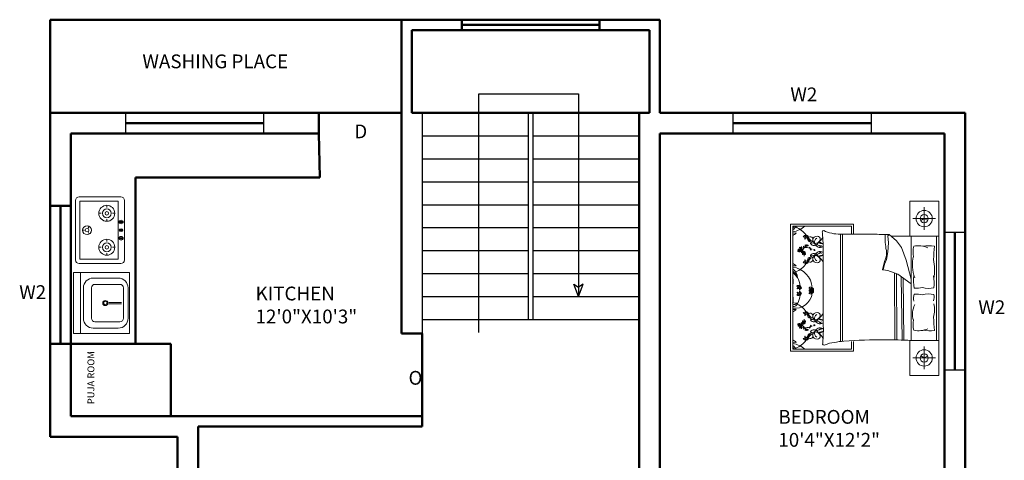
# Model space of a CAD drawing. Units: inches. Extents: x 18 to 447, y -515 to 49.
# Tile 2 of 2: x 18 to 447, y -143 to 49. Entities that reach past the tile are written whole.
import ezdxf

# ---------------------------------------------------------------- set-up
doc = ezdxf.new("R2010")
doc.units = ezdxf.units.IN
doc.header["$MEASUREMENT"] = 0
for name, color, linetype, lineweight in [('A-ANNO-TEXT', 7, 'Continuous', 25), ('A-AREA-IDEN', 3, 'Continuous', 25), ('A-FLOR-FIXT', 9, 'Continuous', 18), ('A-FLOR-STRS', 3, 'Continuous', 25), ('A-FURN', 8, 'Continuous', 18), ('A-GLAZ', 4, 'Continuous', 25), ('A-WALL', 7, 'Continuous', 50)]:
    doc.layers.add(name, color=color, linetype=linetype, lineweight=lineweight)
doc.styles.get("Standard").update_dxf_attribs({"font": 'arial.ttf'})

# ---------------------------------------------------------------- blocks, each defined once
blk = doc.blocks.new('М14 600х655')
for p, q in [((-655, 600), (-655, 0)), ((-655, 600), (-655, 0)), ((-655, 0), (-655, 600)), ((0, 600), (-655, 600)), ((0, 0), (0, 600)), ((0, 525), (-655, 525)), ((-165, 494), (-490, 494)), ((-596, 388), (-596, 121)), ((-528, 370), (-528, 103)), ((-165, 408), (-490, 408)), ((-127, 103), (-127, 370)), ((-59, 121), (-59, 388)), ((-334, 87), (-334, 220)), ((-321, 87), (-321, 220)), ((-655, 0), (-655, 0)), ((-655, 0), (-655, 0)), ((-655, 0), (0, 0)), ((-655, 0), (0, 0)), ((-490, 65), (-165, 65)), ((-490, 15), (-165, 15))]:
    blk.add_line(p, q)
for radius in [27.6, 19.3]:
    blk.add_circle((-327, 259), radius)
for centre, radius, start, end in [((-490, 388), 106, 90, 180), ((-165, 388), 106, 0, 90), ((-490, 370), 38.2, 90, 180), ((-165, 370), 38.2, 0, 90), ((-490, 121), 106, 180, 270), ((-165, 121), 106, 270, 0), ((-490, 103), 38.2, 180, 270), ((-165, 103), 38.2, 270, 0)]:
    blk.add_arc(centre, radius, start, end)
blk = doc.blocks.new('BED-DOUBLE')
for p, q in [((412.28, -42.96), (412.28, -33.06)), ((418.6, -30.43), (418.6, -106.23)), ((407.33, -38.01), (417.24, -38.01)), ((354.14, -40.44), (381.44, -40.44)), ((354.14, -95.69), (354.14, -40.44)), ((355.02, -41.31), (355.02, -94.82)), ((380.57, -41.31), (355.02, -41.31)), ((380.57, -44.72), (380.57, -41.31)), ((381.44, -40.44), (381.44, -44.72)), ((375.77, -91.48), (375.77, -44.72)), ((376.72, -91.41), (376.72, -44.72)), ((396.39, -45.53), (397.01, -44.91)), ((396.7, -48.6), (396.39, -45.53)), ((397.01, -44.91), (400.23, -47.67)), ((418.6, -45.59), (397.8, -45.59)), ((406.62, -45.59), (406.62, -91.07)), ((417.63, -91.07), (417.63, -45.59)), ((362.7, -48.78), (363.56, -48.62)), ((396.39, -52.43), (396.7, -48.6)), ((400.23, -47.67), (402.37, -50.59)), ((402.37, -50.59), (404.37, -56.12)), ((362.7, -54.08), (363.56, -54.25)), ((368.33, -83.72), (368.33, -52.94)), ((395.93, -55.81), (396.39, -52.43)), ((394.4, -60.26), (395.01, -57.81)), ((395.01, -57.81), (395.93, -55.81)), ((404.37, -56.12), (406.62, -64.38)), ((396.39, -60.57), (394.4, -60.26)), ((400.84, -62.26), (396.39, -60.57)), ((399.53, -90.8), (399.41, -61.72)), ((400.31, -90.8), (400.19, -62.01)), ((406.62, -66.41), (400.84, -62.26)), ((402.7, -90.83), (402.31, -63.31)), ((403.47, -90.86), (403.1, -63.88)), ((362.7, -82.05), (363.56, -81.88)), ((362.7, -87.35), (363.56, -87.51)), ((380.57, -94.82), (380.57, -91.47)), ((381.44, -91.49), (381.44, -95.69)), ((412.28, -93.7), (412.28, -103.6)), ((381.44, -95.69), (354.14, -95.69)), ((355.02, -94.82), (380.57, -94.82)), ((407.33, -98.65), (417.24, -98.65))]:
    blk.add_line(p, q)
for points in [[(405.97, -45.59), (405.97, -30.43), (418.6, -30.43)], [(412.28, -38.01), (410.75, -38.89)], [(412.28, -38.01), (413.82, -38.89)], [(418.6, -91.07), (405.97, -91.07), (405.97, -106.23), (418.6, -106.23)], [(412.28, -98.65), (410.75, -97.76)], [(412.28, -98.65), (413.82, -97.76)]]:
    blk.add_lwpolyline(points)
for points in [[(390.06, -44.75, 0.001242), (375.68, -44.72, -0.127202), (368.52, -43.2)], [(416.71, -49.94, 0.074897), (411.76, -50.04, -0.472817)], [(411.48, -67.97, 0.14099), (416.53, -68.13, 0.235245)], [(411.48, -71.21, -0.14099), (416.53, -71.06, -0.235245)], [(416.71, -86.71, -0.074897), (411.76, -86.62, 0.472817)], [(377.31, -91.39, 0.056112), (373.14, -91.94, 0.095341), (369.13, -93.01)]]:
    blk.add_lwpolyline(points, format="xyb")
for centre, radius in [((412.28, -38.01), 3.54), ((412.28, -38.01), 1.77), ((357.92, -51.9), 0.193), ((359.96, -53.16), 0.193), ((357.92, -84.23), 0.193), ((359.96, -82.97), 0.193), ((412.28, -98.65), 3.54), ((412.28, -98.65), 1.77)]:
    blk.add_circle(centre, radius)
for centre, radius, start, end in [((351.46, -37.17), 6.01, 306.3036, 316.4814), ((352.36, -38.91), 4.82, 303.4617, 330.1116), ((353.69, -33.94), 9.9, 277.745, 311.8856), ((352.71, -50.88), 9.9, 34.3865, 68.5908), ((353.48, -41.61), 4.02, 292.5547, 318.9546), ((355.64, -30.59), 13.69, 267.4081, 273.6519), ((360.64, -46.36), 1.1, 77.7115, 159.0387), ((360.05, -45.26), 0.827, 238.4633, 358.2869), ((362.76, -46.94), 2.5, 138.8402, 177.9352), ((360.38, -46.85), 0.123, 177.9352, 11.4834), ((360.44, -46.84), 0.0597, 11.4834, 127.9409), ((361.25, -46.01), 0.81, 117.6827, 223.7762), ((360.74, -46.49), 0.107, 223.7762, 159.7183), ((361.07, -46.09), 0.821, 2.9516, 103.728), ((367.63, -43.79), 6.92, 192.5173, 207.1824), ((359.96, -46.56), 1.56, 345.4653, 54.2343), ((362.32, -44.41), 1.69, 211.3827, 255.2969), ((362.98, -46.78), 1.42, 175.969, 254.3045), ((362.64, -47.05), 1.14, 350.264, 160.8688), ((361.41, -46.82), 0.697, 333.9755, 53.2681), ((361.1, -48.31), 1.51, 6.1662, 51.5825), ((365.15, -44.79), 3.58, 211.2614, 251.7045), ((365.56, -47.47), 1.81, 84.9449, 172.8857), ((366.25, -48.18), 1.76, 111.5819, 201.4221), ((364.8, -46.55), 2.28, 265.2933, 346.921), ((365.74, -46.94), 1.28, 354.4856, 91.0538), ((362.99, -43.6), 5.74, 303.6671, 333.2997), ((368.56, -43.89), 0.699, 93.98, 207.3412), ((289.43, -52.04), 78.9, 359.3433, 5.6887), ((395.12, 24.59), 69.52, 265.8294, 271.553), ((423.85, -46.21), 28.61, 177.4519, 191.3392), ((357.77, -51.51), 0.381, 157.4086, 261.4386), ((357.56, -51.49), 0.191, 58.0499, 135.6268), ((357.34, -51.85), 0.609, 14.7558, 58.0499), ((358.19, -51.69), 0.263, 36.1046, 181.4281), ((358.2, -50.65), 0.216, 124.3538, 214.3923), ((358.52, -50.69), 0.503, 190.3057, 287.1958), ((358.66, -50.51), 0.583, 176.9701, 248.2913), ((362.83, -47.43), 5.64, 212.6784, 216.3746), ((358.47, -50.64), 0.223, 216.3746, 291.7548), ((360.44, -53.78), 3.15, 124.0033, 132.4917), ((357.21, -54.17), 3.36, 63.7819, 68.2913), ((359, -51.59), 0.535, 128.3208, 208.8162), ((359, -50.8), 0.503, 122.8155, 187.3992), ((358.61, -51.01), 0.168, 289.3605, 111.7548), ((358.74, -51.01), 0.168, 221.8703, 44.2646), ((359.5, -51.5), 0.88, 157.2305, 229.0635), ((359.22, -50.86), 0.583, 109.4799, 177.6828), ((359.21, -51.21), 0.518, 174.4544, 220.6188), ((356.26, -54.1), 3.78, 30.544, 49.818), ((358.91, -50.49), 0.216, 56.8636, 146.9021), ((359.02, -50.73), 0.223, 148.8844, 224.2646), ((363.66, -53.53), 5.64, 145.1882, 148.8844), ((360.44, -53.78), 3.15, 94.756, 119.2041), ((367.14, -58.31), 10.36, 132.2412, 142.1744), ((361.92, -50.06), 2.14, 178.3264, 187.1302), ((359.61, -50.36), 0.398, 11.3256, 64.4621), ((360.96, -49.79), 1.2, 190.2588, 210.656), ((360.15, -50.28), 0.364, 188.3432, 274.2869), ((360.47, -50.07), 0.635, 210.656, 242.6341), ((360.95, -49.53), 1.22, 218.2101, 226.3071), ((360.05, -50.55), 0.154, 325.7657, 67.4417), ((355.26, -45.39), 7.2, 313.1541, 322.0459), ((360.6, -56.9), 6.28, 73.5842, 93.8277), ((360.55, -49.71), 0.148, 142.4737, 265.053), ((360.75, -49.68), 0.319, 127.7621, 169.0403), ((360.58, -49.41), 0.449, 265.053, 338.3618), ((361.17, -50.03), 0.586, 113.4276, 137.6104), ((361.1, -49.42), 0.193, 183.2768, 356.7232), ((361.25, -49.77), 0.316, 139.7889, 227.6792), ((361.15, -49.88), 0.166, 227.6792, 350.3487), ((360.5, -49.76), 0.632, 353.0852, 15.7171), ((360.92, -49.84), 0.399, 350.3487, 43.6538), ((361.66, -49.43), 0.464, 198.7263, 262.5032), ((361.29, -49.64), 0.184, 1.1081, 91.8675), ((361.63, -49.74), 0.149, 255.2356, 54.9248), ((361.4, -49.69), 0.322, 11.5637, 52.6358), ((364.47, -50.52), 2.14, 178.3264, 187.1302), ((362.16, -50.81), 0.398, 11.3256, 64.4621), ((363.51, -50.24), 1.2, 190.2588, 210.656), ((362.7, -50.73), 0.364, 188.3432, 274.2869), ((363.02, -50.53), 0.635, 210.656, 242.6341), ((363.5, -49.98), 1.22, 218.2101, 226.3071), ((364.86, -44.76), 4.07, 236.2883, 266.5076), ((362.6, -51), 0.154, 325.7657, 67.4417), ((363.04, -51.29), 0.364, 147.5332, 233.4768), ((364.34, -47.84), 1.88, 209.9085, 343.1337), ((363.37, -51.1), 0.635, 179.1859, 211.164), ((362.75, -51.24), 0.154, 354.3784, 96.0543), ((360.6, -56.9), 6.28, 63.0032, 69.8941), ((363.85, -50.81), 1.2, 211.164, 231.5612), ((364.07, -50.93), 1.22, 195.5129, 203.6099), ((362.71, -51.73), 0.398, 357.3579, 50.4944), ((365.96, -47.15), 2.2, 182.3591, 234.0401), ((365.13, -49.04), 0.47, 167.3041, 285.1471), ((366.4, -51.29), 2.92, 122.7011, 126.3445), ((366.95, -48.14), 2.42, 199.2822, 299.1751), ((365.66, -50.99), 1.55, 41.5653, 105.1471), ((367.77, -45.7), 3.14, 238.8218, 279.1554), ((366.4, -51.29), 2.92, 55.785, 94.7304), ((366.51, -47.77), 2.18, 277.436, 299.9149), ((367.67, -49.21), 1.13, 221.5653, 293.8354), ((367.49, -49.59), 0.913, 30.0293, 52.325), ((367.49, -49.59), 0.913, 314.4517, 333.558), ((417.6, -52.65), 10.16, 165.1039, 191.0369), ((409.77, -59.6), 9.77, 65.1316, 101.7583), ((1138.04, -91.72), 722.54, 176.68521, 177.14978), ((357.37, -52.19), 0.148, 142.4737, 265.053), ((357.56, -52.16), 0.319, 61.2196, 169.0403), ((357.4, -51.89), 0.449, 265.053, 338.3618), ((357.99, -52.51), 0.586, 113.4276, 137.6104), ((357.76, -51.61), 0.128, 172.906, 277.132), ((358.06, -52.25), 0.316, 139.7889, 227.6792), ((357.96, -52.36), 0.166, 227.6792, 350.3487), ((357.32, -52.24), 0.632, 353.0852, 15.7171), ((357.73, -52.32), 0.399, 350.3487, 43.6538), ((358.47, -51.91), 0.464, 198.7263, 262.5032), ((358.04, -51.48), 0.266, 270.0645, 331.1507), ((358.26, -51.54), 0.304, 221.8413, 265.7877), ((358.1, -52.12), 0.184, 1.1081, 91.8675), ((358.26, -51.66), 0.189, 263.7526, 41.7054), ((358.22, -52.17), 0.322, 11.5637, 86.365), ((358.45, -52.22), 0.149, 255.2356, 54.9248), ((359.1, -51.55), 0.639, 207.7043, 254.3516), ((358.68, -51.91), 0.88, 270.278, 342.111), ((359.27, -53.01), 0.622, 98.7227, 159.3375), ((358.96, -52.21), 0.639, 244.9899, 291.6373), ((358.34, -51.95), 0.622, 340.0041, 40.6188), ((359.1, -51.89), 0.518, 278.7227, 324.8872), ((359, -52.31), 0.535, 290.5253, 358.5375), ((359.4, -53.45), 0.148, 142.4737, 265.053), ((359.6, -53.42), 0.319, 61.2196, 169.0403), ((359.43, -53.16), 0.449, 265.053, 338.3618), ((359.81, -52.77), 0.381, 157.4086, 261.4386), ((359.59, -52.76), 0.191, 58.0499, 135.6268), ((360.05, -52.15), 0.535, 182.8499, 266.1226), ((359.84, -51.78), 0.518, 231.7607, 277.9252), ((360.24, -51.68), 0.88, 214.5369, 286.3699), ((360.02, -53.77), 0.586, 113.4276, 137.6104), ((359.79, -52.88), 0.128, 172.906, 277.132), ((359.37, -53.11), 0.609, 14.7558, 58.0499), ((356.26, -54.1), 3.78, 23.0501, 23.8477), ((360.1, -53.51), 0.316, 139.7889, 227.6792), ((360, -53.62), 0.166, 227.6792, 350.3487), ((360, -52.91), 0.622, 37.3105, 97.9252), ((360.23, -52.95), 0.263, 36.1046, 181.4281), ((359.35, -53.51), 0.632, 353.0852, 15.7171), ((360.07, -52.05), 0.639, 265.0106, 311.658), ((356.26, -54.1), 3.78, 357.1071, 4.7585), ((359.77, -53.58), 0.399, 350.3487, 43.6538), ((360.07, -52.74), 0.266, 270.0645, 331.1507), ((360.3, -52.8), 0.304, 221.8413, 265.7877), ((360.51, -53.17), 0.464, 198.7263, 262.5032), ((360.14, -53.39), 0.184, 1.1081, 91.8675), ((360.3, -52.92), 0.189, 263.7526, 41.7054), ((360.26, -53.43), 0.322, 11.5637, 86.365), ((360.49, -53.49), 0.149, 255.2356, 54.9248), ((362.98, -56.09), 1.42, 105.6955, 184.031), ((362.64, -55.81), 1.14, 199.1312, 9.736), ((361.1, -54.56), 1.51, 308.4175, 353.8338), ((365.15, -58.07), 3.58, 108.2955, 148.7386), ((364.86, -58.1), 4.07, 93.4924, 123.7117), ((364.34, -55.02), 1.88, 16.8663, 150.0915), ((364.06, -49.83), 2.14, 234.6898, 243.4936), ((365.96, -55.71), 2.2, 125.9599, 177.6409), ((365.56, -55.4), 1.81, 187.1143, 275.0551), ((364.42, -51.65), 0.146, 12.7051, 190.4384), ((364.51, -51.63), 0.238, 190.4384, 10.4136), ((366.25, -54.69), 1.76, 158.5779, 248.4181), ((364.8, -56.31), 2.28, 13.079, 94.7067), ((365.13, -53.83), 0.47, 74.8529, 192.6959), ((366.95, -54.73), 2.42, 60.8249, 160.7178), ((366.4, -51.58), 2.92, 233.6555, 237.2989), ((365.66, -51.87), 1.55, 254.8529, 318.4347), ((367.77, -57.16), 3.14, 79.7133, 121.1782), ((366.4, -51.58), 2.92, 265.2696, 304.215), ((362.99, -59.26), 5.74, 21.4941, 56.3329), ((366.51, -55.09), 2.18, 60.0851, 82.564), ((367.67, -53.66), 1.13, 66.1646, 138.4347), ((367.49, -53.27), 0.913, 307.675, 336.7144), ((367.49, -53.27), 0.913, 23.229, 45.5483), ((423.04, -65.53), 29.39, 160.1194, 169.3383), ((389.75, -53.05), 6.17, 336.2616, 11.3392), ((424.82, -57.99), 17.62, 168.0397, 199.2615), ((353.48, -61.25), 4.02, 41.0454, 67.4453), ((355.64, -72.28), 13.69, 86.3481, 92.5919), ((353.69, -68.92), 9.9, 4.4623, 82.255), ((352.36, -63.95), 4.82, 1.272, 56.5383), ((352.71, -51.98), 9.9, 291.4092, 325.6135), ((360.05, -57.6), 0.827, 1.7131, 121.5367), ((360.64, -56.5), 1.1, 200.9613, 282.2885), ((360.38, -56.01), 0.123, 348.5166, 182.0648), ((362.76, -55.93), 2.5, 182.0648, 221.1598), ((360.44, -56.03), 0.0597, 232.0591, 348.5166), ((361.25, -56.86), 0.81, 136.2238, 242.3173), ((360.78, -56.38), 0.0645, 200.2667, 136.2271), ((359.96, -56.3), 1.56, 305.7657, 14.5347), ((367.63, -59.08), 6.92, 152.8176, 167.4827), ((361.07, -56.78), 0.821, 256.272, 357.0484), ((362.32, -58.45), 1.69, 104.7031, 148.6173), ((361.41, -56.05), 0.697, 306.7319, 26.0245), ((365.74, -55.92), 1.28, 268.9462, 5.5144), ((389.28, -60.33), 27.49, 352.2196, 9.497), ((351.46, -65.69), 6.01, 17.8504, 53.6964), ((349.77, -68.85), 8.94, 34.0123, 54.053), ((349.81, -65.39), 5.44, 343.5431, 17.0202), ((348.38, -68.16), 9.9, 4.4623, 27.4146), ((394.34, -60.09), 0.183, 178.8623, 289.7536), ((420.97, -65.13), 13.37, 169.8617, 193.6238), ((403.18, -66.14), 13.51, 351.5249, 13.96), ((347.01, -67.55), 8.05, 4.3787, 5.6357), ((341.5, -71.79), 14.38, 19.7217, 19.9028), ((357.51, -68.2), 1.1, 47.7873, 129.1145), ((357.55, -66.96), 0.827, 208.5391, 328.3627), ((357.04, -68.5), 0.123, 148.011, 341.5592), ((359.06, -69.76), 2.5, 108.9159, 148.011), ((357.1, -68.52), 0.0597, 341.5592, 98.0167), ((358.22, -68.2), 0.81, 87.7585, 193.852), ((357.54, -68.37), 0.107, 193.852, 129.9245), ((364.86, -69.46), 6.92, 162.593, 177.2582), ((356.83, -68.03), 1.56, 315.5411, 24.3101), ((359.94, -67.35), 1.69, 181.4585, 225.3727), ((358.02, -68.18), 0.821, 333.0274, 73.8037), ((362.82, -68.96), 1.1, 47.7873, 129.1145), ((362.85, -67.71), 0.827, 208.5391, 328.3627), ((364.36, -70.52), 2.5, 108.9159, 148.011), ((363.52, -68.96), 0.81, 87.7585, 193.852), ((362.13, -68.79), 1.56, 315.5411, 24.3101), ((370.16, -70.22), 6.92, 162.593, 177.2582), ((363.32, -68.94), 0.821, 333.0274, 73.8037), ((365.24, -68.11), 1.69, 181.4585, 225.3727), ((408.95, -59.04), 9.29, 264.0129, 285.8293), ((355.97, -69.42), 7.66, 262.8636, 351.8197), ((349.81, -73.26), 5.44, 342.9798, 16.4569), ((347.01, -71.11), 8.05, 354.3643, 355.6213), ((341.5, -66.87), 14.38, 340.0972, 340.2783), ((357.55, -71.7), 0.827, 31.6373, 151.4609), ((357.51, -70.45), 1.1, 230.8855, 312.2127), ((357.04, -70.16), 0.123, 18.4408, 211.989), ((359.06, -68.9), 2.5, 211.989, 251.0841), ((357.1, -70.14), 0.0597, 261.9833, 18.4408), ((348.38, -70.5), 9.9, 332.5854, 355.5377), ((358.22, -70.46), 0.81, 166.148, 272.2415), ((357.58, -70.28), 0.0645, 230.1909, 166.0209), ((364.86, -69.19), 6.92, 182.7418, 197.407), ((356.83, -70.62), 1.56, 335.6899, 44.4589), ((359.94, -71.31), 1.69, 134.6273, 178.5415), ((358.02, -70.48), 0.821, 286.1963, 26.9726), ((362.85, -70.94), 0.827, 31.6373, 151.4609), ((362.82, -69.69), 1.1, 230.8855, 312.2127), ((362.35, -69.26), 0.123, 148.011, 341.5592), ((362.35, -69.4), 0.123, 18.4408, 211.989), ((364.36, -68.14), 2.5, 211.989, 251.0841), ((362.41, -69.28), 0.0597, 341.5592, 98.0167), ((362.41, -69.38), 0.0597, 261.9833, 18.4408), ((363.52, -69.7), 0.81, 166.148, 272.2415), ((362.84, -69.13), 0.107, 193.852, 129.9245), ((362.88, -69.52), 0.0645, 230.1909, 166.0209), ((362.13, -69.86), 1.56, 335.6899, 44.4589), ((370.16, -68.44), 6.92, 182.7418, 197.407), ((363.32, -69.72), 0.821, 286.1963, 26.9726), ((365.24, -70.55), 1.69, 134.6273, 178.5415), ((411.62, -72.61), 4.02, 155.0183, 198.5407), ((408.95, -80.15), 9.29, 74.1707, 95.9871), ((412.93, -72.1), 3.75, 333.3437, 16.1026), ((356.67, -70.41), 4.43, 248.117, 276.6195), ((355.44, -74.47), 1.78, 256.3898, 349.0739), ((355.68, -73.14), 2.25, 252.8609, 311.9049), ((352.71, -84.14), 9.9, 34.3865, 68.5908), ((416.85, -79.63), 9.65, 153.8761, 196.1746), ((403.45, -77.72), 13.32, 346.3427, 11.1841), ((355.64, -63.85), 13.69, 267.4081, 273.6519), ((353.48, -74.88), 4.02, 292.5547, 318.9546), ((360.64, -79.63), 1.1, 77.7115, 159.0387), ((360.05, -78.53), 0.827, 238.4633, 358.2869), ((362.76, -80.2), 2.5, 138.8402, 177.9352), ((360.38, -80.12), 0.123, 177.9352, 11.4834), ((360.44, -80.1), 0.0597, 11.4834, 127.9409), ((361.25, -79.27), 0.81, 117.6827, 223.7762), ((360.74, -79.76), 0.107, 223.7762, 159.7183), ((361.07, -79.35), 0.821, 2.9516, 103.728), ((362.32, -77.67), 1.69, 211.3827, 255.2969), ((359.96, -79.82), 1.56, 345.4653, 54.2343), ((367.63, -77.05), 6.92, 192.5173, 207.1824), ((362.98, -80.04), 1.42, 175.969, 254.3045), ((362.64, -80.32), 1.14, 350.264, 160.8688), ((361.41, -80.08), 0.697, 333.9755, 53.2681), ((361.1, -81.57), 1.51, 6.1662, 51.5825), ((365.15, -78.06), 3.58, 211.2614, 251.7045), ((364.86, -78.03), 4.07, 236.2883, 266.5076), ((365.56, -80.73), 1.81, 84.9449, 172.8857), ((365.96, -80.42), 2.2, 182.3591, 234.0401), ((366.25, -81.44), 1.76, 111.5819, 201.4221), ((364.8, -79.81), 2.28, 265.2933, 346.921), ((365.74, -80.21), 1.28, 354.4856, 91.0538), ((362.99, -76.87), 5.74, 303.6671, 338.5059), ((1138.04, -44.94), 722.54, 182.85022, 183.31479), ((357.37, -83.94), 0.148, 94.947, 217.5263), ((357.56, -83.97), 0.319, 190.9597, 298.7804), ((357.4, -84.24), 0.449, 21.6382, 94.947), ((357.77, -84.62), 0.381, 98.5614, 202.5914), ((357.56, -84.64), 0.191, 224.3732, 301.9501), ((357.99, -83.62), 0.586, 222.3896, 246.5724), ((357.76, -84.52), 0.128, 82.868, 187.094), ((357.34, -84.28), 0.609, 301.9501, 345.2442), ((358.06, -83.88), 0.316, 132.3208, 220.2111), ((357.96, -83.77), 0.166, 9.6513, 132.3208), ((357.32, -83.88), 0.632, 344.2829, 6.9148), ((358.19, -84.44), 0.263, 178.5719, 323.8954), ((358.2, -85.47), 0.216, 145.6077, 235.6462), ((357.73, -83.81), 0.399, 316.3462, 9.6513), ((358.47, -84.22), 0.464, 97.4968, 161.2737), ((358.52, -85.44), 0.503, 72.8042, 169.6943), ((358.26, -84.59), 0.304, 94.2123, 138.1587), ((358.04, -84.65), 0.266, 28.8493, 89.9355), ((358.66, -85.62), 0.583, 111.7087, 183.0299), ((362.83, -88.7), 5.64, 143.6254, 147.3216), ((358.1, -84), 0.184, 268.1325, 358.8919), ((358.22, -83.96), 0.322, 273.635, 348.4363), ((358.26, -84.47), 0.189, 318.2946, 96.2474), ((358.47, -85.49), 0.223, 68.2452, 143.6254), ((360.44, -82.35), 3.15, 227.5083, 235.9967), ((358.45, -83.91), 0.149, 305.0752, 104.7644), ((357.21, -81.96), 3.36, 291.7087, 296.2181), ((359, -84.54), 0.535, 151.1838, 231.6792), ((359, -85.33), 0.503, 172.6008, 237.1845), ((359.1, -84.58), 0.639, 105.6484, 152.2957), ((358.61, -85.12), 0.168, 248.2452, 70.6395), ((358.74, -85.12), 0.168, 315.7354, 138.1297), ((359.5, -84.63), 0.88, 130.9365, 202.7695), ((359.22, -85.26), 0.583, 182.3172, 250.5201), ((358.96, -83.92), 0.639, 68.3627, 115.0101), ((358.68, -84.22), 0.88, 17.889, 89.722), ((359.27, -83.12), 0.622, 200.6625, 261.2773), ((359.21, -84.92), 0.518, 139.3812, 185.5456), ((356.26, -82.03), 3.78, 310.182, 329.456), ((359.02, -85.39), 0.223, 135.7354, 211.1156), ((358.34, -84.18), 0.622, 319.3812, 19.9959), ((363.66, -82.6), 5.64, 211.1156, 214.8118), ((360.44, -82.35), 3.15, 240.7959, 265.244), ((367.14, -77.82), 10.36, 217.8256, 227.7588), ((359.1, -84.24), 0.518, 35.1128, 81.2773), ((359, -83.82), 0.535, 1.4625, 69.4747), ((359.4, -82.67), 0.148, 94.947, 217.5263), ((359.6, -82.7), 0.319, 190.9597, 298.7804), ((359.43, -82.97), 0.449, 21.6382, 94.947), ((359.81, -83.36), 0.381, 98.5614, 202.5914), ((359.59, -83.37), 0.191, 224.3732, 301.9501), ((360.05, -83.98), 0.535, 93.8774, 177.1501), ((360.24, -84.44), 0.88, 73.6301, 145.4631), ((359.84, -84.35), 0.518, 82.0748, 128.2393), ((360.02, -82.36), 0.586, 222.3896, 246.5724), ((359.79, -83.25), 0.128, 82.868, 187.094), ((359.37, -83.02), 0.609, 301.9501, 345.2442), ((356.26, -82.03), 3.78, 336.1523, 336.9499), ((360.1, -82.62), 0.316, 132.3208, 220.2111), ((360.96, -86.34), 1.2, 149.344, 169.7412), ((360.15, -85.85), 0.364, 85.7131, 171.6568), ((360, -82.51), 0.166, 9.6513, 132.3208), ((360, -83.22), 0.622, 262.0748, 322.6895), ((360.47, -86.05), 0.635, 117.3659, 149.344), ((359.35, -82.62), 0.632, 344.2829, 6.9148), ((360.23, -83.18), 0.263, 178.5719, 323.8954), ((360.95, -86.6), 1.22, 133.6929, 141.7899), ((360.07, -84.08), 0.639, 48.342, 94.9894), ((356.26, -82.03), 3.78, 355.2415, 2.8929), ((359.77, -82.55), 0.399, 316.3462, 9.6513), ((360.51, -82.96), 0.464, 97.4968, 161.2737), ((360.3, -83.32), 0.304, 94.2123, 138.1587), ((360.07, -83.39), 0.266, 28.8493, 89.9355), ((360.05, -85.58), 0.154, 292.5583, 34.2343), ((360.14, -82.74), 0.184, 268.1325, 358.8919), ((360.6, -79.23), 6.28, 266.1723, 286.4158), ((355.26, -90.74), 7.2, 37.9541, 46.8459), ((360.26, -82.7), 0.322, 273.635, 348.4363), ((360.3, -83.21), 0.189, 318.2946, 96.2474), ((360.49, -82.64), 0.149, 305.0752, 104.7644), ((363.51, -85.89), 1.2, 149.344, 169.7412), ((364.47, -85.61), 2.14, 172.8698, 181.6736), ((362.16, -85.32), 0.398, 295.5379, 348.6744), ((362.7, -85.4), 0.364, 85.7131, 171.6568), ((363.02, -85.6), 0.635, 117.3659, 149.344), ((363.5, -86.15), 1.22, 133.6929, 141.7899), ((362.6, -85.13), 0.154, 292.5583, 34.2343), ((363.04, -84.84), 0.364, 126.5232, 212.4668), ((364.34, -81.11), 1.88, 209.9085, 343.1337), ((363.37, -85.03), 0.635, 148.836, 180.8141), ((362.75, -84.88), 0.154, 263.9457, 5.6216), ((360.6, -79.23), 6.28, 290.1059, 296.9968), ((363.85, -85.32), 1.2, 128.4388, 148.836), ((364.06, -86.3), 2.14, 116.5064, 125.3102), ((364.07, -85.2), 1.22, 156.3901, 164.4871), ((362.71, -84.4), 0.398, 309.5056, 2.6421), ((364.51, -84.5), 0.238, 349.5864, 169.5616), ((364.42, -84.48), 0.146, 169.5616, 347.2949), ((365.13, -82.3), 0.47, 167.3041, 285.1471), ((366.4, -84.55), 2.92, 122.7011, 126.3445), ((366.95, -81.4), 2.42, 199.2822, 299.1751), ((366.95, -87.99), 2.42, 60.8249, 160.7178), ((365.66, -84.26), 1.55, 41.5653, 105.1471), ((367.77, -78.97), 3.14, 238.8218, 280.2867), ((366.4, -84.55), 2.92, 55.785, 94.7304), ((366.51, -81.04), 2.18, 277.436, 299.9149), ((367.67, -82.47), 1.13, 221.5653, 293.8354), ((367.49, -82.86), 0.913, 23.2856, 52.325), ((294.61, -86.04), 73.76, 355.2402, 1.8035), ((367.49, -82.86), 0.913, 314.4517, 336.7144), ((417.6, -84.01), 10.16, 168.9631, 194.8961), ((358.91, -85.63), 0.216, 213.0979, 303.1364), ((361.92, -86.07), 2.14, 172.8698, 181.6736), ((359.61, -85.77), 0.398, 295.5379, 348.6744), ((360.38, -89.28), 0.123, 348.5166, 182.0648), ((362.76, -89.19), 2.5, 182.0648, 221.1598), ((360.55, -86.42), 0.148, 94.947, 217.5263), ((360.44, -89.29), 0.0597, 232.0591, 348.5166), ((360.75, -86.45), 0.319, 190.9597, 232.2379), ((361.25, -90.12), 0.81, 136.2238, 242.3173), ((360.58, -86.72), 0.449, 21.6382, 94.947), ((360.78, -89.65), 0.0645, 200.2667, 136.2271), ((361.17, -86.1), 0.586, 222.3896, 246.5724), ((367.63, -92.34), 6.92, 152.8176, 167.4827), ((359.96, -89.57), 1.56, 305.7657, 14.5347), ((361.1, -86.71), 0.193, 3.2768, 176.7232), ((361.25, -86.36), 0.316, 132.3208, 220.2111), ((361.15, -86.25), 0.166, 9.6513, 132.3208), ((360.5, -86.36), 0.632, 344.2829, 6.9148), ((360.92, -86.29), 0.399, 316.3462, 9.6513), ((361.66, -86.7), 0.464, 97.4968, 161.2737), ((361.29, -86.48), 0.184, 268.1325, 358.8919), ((362.98, -89.35), 1.42, 105.6955, 184.031), ((362.64, -89.08), 1.14, 199.1312, 9.736), ((361.63, -86.38), 0.149, 305.0752, 104.7644), ((361.4, -86.44), 0.322, 307.3642, 348.4363), ((361.41, -89.31), 0.697, 306.7319, 26.0245), ((361.1, -87.82), 1.51, 308.4175, 353.8338), ((365.15, -91.34), 3.58, 108.2955, 148.7386), ((364.86, -91.37), 4.07, 93.4924, 123.7117), ((364.34, -88.29), 1.88, 16.8663, 150.0915), ((365.96, -88.98), 2.2, 125.9599, 177.6409), ((365.56, -88.66), 1.81, 187.1143, 275.0551), ((366.25, -87.95), 1.76, 158.5779, 248.4181), ((364.8, -89.58), 2.28, 13.079, 94.7067), ((365.13, -87.09), 0.47, 74.8529, 192.6959), ((366.4, -84.84), 2.92, 233.6555, 237.2989), ((365.66, -85.14), 1.55, 254.8529, 318.4347), ((365.74, -89.19), 1.28, 268.9462, 5.5144), ((367.77, -90.43), 3.14, 79.249, 121.1782), ((366.4, -84.84), 2.92, 265.2696, 304.215), ((362.99, -92.53), 5.74, 23.6453, 56.3329), ((366.51, -88.36), 2.18, 60.0851, 82.564), ((367.67, -86.92), 1.13, 66.1646, 138.4347), ((367.49, -86.54), 0.913, 307.675, 342.5814), ((367.49, -86.54), 0.913, 16.6343, 45.5483), ((409.77, -77.06), 9.77, 258.2417, 294.8684), ((353.48, -94.52), 4.02, 41.0454, 67.4453), ((355.64, -105.54), 13.69, 86.3481, 92.5919), ((353.69, -102.18), 9.9, 48.1144, 82.255), ((352.36, -97.22), 4.82, 29.8884, 56.5383), ((351.46, -98.95), 6.01, 43.5186, 53.6964), ((352.71, -85.25), 9.9, 291.4092, 325.6135), ((360.05, -90.87), 0.827, 1.7131, 121.5367), ((360.64, -89.77), 1.1, 200.9613, 282.2885), ((362.32, -91.72), 1.69, 104.7031, 148.6173), ((361.07, -90.04), 0.821, 256.272, 357.0484), ((368.74, -92.43), 0.691, 156.5219, 303.8264), ((392.41, -268.41), 177.66, 89.1145, 94.8735), ((397.36, -226.95), 136.19, 86.1, 90.9282)]:
    blk.add_arc(centre, radius, start, end)
blk = doc.blocks.new('WIN-W')
for p, q in [((0, 9), (60, 9)), ((0, 0), (0, 9)), ((60, 9), (60, 0)), ((60, 0), (0, 0))]:
    blk.add_line(p, q)

msp = doc.modelspace()

# ---------------------------------------------------------------- linework, layer by layer
at = {"layer": 'A-FLOR-FIXT'}
for p, q in [((44.32, -28.55), (62.5, -28.55)), ((42.77, -56.02), (42.77, -30.1)), ((44.7, -55.63), (44.7, -30.48)), ((44.7, -30.48), (61.34, -30.48)), ((56.39, -32.23), (56.39, -33.19)), ((61.34, -30.48), (61.34, -55.63)), ((64.05, -30.1), (64.05, -56.02)), ((52.9, -35.71), (53.87, -35.71)), ((56.39, -38.22), (56.39, -39.19)), ((58.9, -35.71), (59.87, -35.71)), ((48.65, -41.32), (48.28, -42)), ((61.64, -39.3), (63.57, -39.3)), ((61.64, -39.69), (63.57, -39.69)), ((45.87, -43.06), (46.64, -43.06)), ((48.65, -44.8), (48.36, -44.08)), ((56.39, -47.01), (56.39, -47.98)), ((61.64, -46.38), (63.57, -46.38)), ((61.64, -46.77), (63.57, -46.77)), ((61.82, -42.89), (63.38, -42.89)), ((61.82, -43.2), (63.38, -43.2)), ((52.9, -50.49), (53.87, -50.49)), ((58.9, -50.49), (59.87, -50.49)), ((61.34, -55.63), (44.7, -55.63)), ((56.39, -53.01), (56.39, -53.98)), ((62.5, -57.57), (44.32, -57.57))]:
    msp.add_line(p, q, dxfattribs=at)
for centre, radius in [((56.39, -35.71), 3.48), ((56.39, -35.71), 1.93), ((56.39, -35.71), 0.774), ((47.8, -43.06), 1.93), ((47.8, -43.06), 0.774), ((56.39, -50.49), 3.48), ((56.39, -50.49), 1.93), ((56.39, -50.49), 0.774)]:
    msp.add_circle(centre, radius, dxfattribs=at)
for centre, start, end in [((44.32, -30.1), 90, 180), ((62.5, -30.1), 0, 90), ((44.32, -56.02), 180, 270), ((62.5, -56.02), 270, 0)]:
    msp.add_arc(centre, 1.55, start, end, dxfattribs=at)
for centre, major_axis in [((62.6, -39.49), (0.967, 0)), ((62.6, -43.04), (0.784, 0)), ((62.6, -46.58), (0.967, 0))]:
    msp.add_ellipse(centre, major_axis=major_axis, ratio=0.802399, dxfattribs=at)
at = {"layer": 'A-FLOR-STRS'}
for p, q in [((218.35, -87.63), (218.35, 16.34)), ((218.35, 16.34), (261.77, 16.34)), ((261.77, 16.34), (261.77, -71.95)), ((193.66, 8.05), (193.66, -87.95)), ((239.91, 8.05), (239.91, -81.95)), ((241.91, 8.05), (241.91, -81.95)), ((193.66, -1.95), (239.91, -1.95)), ((241.91, -1.95), (288.17, -1.95)), ((193.66, -11.95), (239.91, -11.95)), ((241.91, -11.95), (288.17, -11.95)), ((193.66, -21.95), (239.91, -21.95)), ((241.91, -21.95), (288.17, -21.95)), ((193.66, -31.95), (239.91, -31.95)), ((241.91, -31.95), (288.17, -31.95)), ((193.66, -41.95), (239.91, -41.95)), ((241.91, -41.95), (288.17, -41.95)), ((193.66, -51.95), (239.91, -51.95)), ((241.91, -51.95), (288.17, -51.95)), ((241.91, -51.95), (288.17, -51.95)), ((193.66, -61.95), (239.91, -61.95)), ((241.91, -61.95), (288.17, -61.95)), ((261.77, -71.95), (259.68, -66.51)), ((259.68, -66.51), (261.77, -67.87)), ((261.77, -71.95), (263.86, -66.51)), ((263.86, -66.51), (261.77, -67.87)), ((193.66, -71.95), (239.91, -71.95)), ((241.91, -71.95), (288.17, -71.95)), ((193.66, -81.95), (241.91, -81.95)), ((241.91, -81.95), (288.17, -81.95))]:
    msp.add_line(p, q, dxfattribs=at)
at = {"layer": 'A-WALL'}
for p, q in [((184.66, 48.55), (31.66, 48.55)), ((31.66, 48.55), (31.66, 8.05)), ((184.66, 48.55), (184.66, -87.95)), ((184.66, 48.55), (297.17, 48.55)), ((210.91, 48.55), (270.91, 48.55)), ((210.91, 44.05), (210.91, 48.55)), ((270.91, 48.55), (270.91, 44.05)), ((297.17, 48.55), (297.17, 8.05)), ((189.16, 44.05), (189.16, 8.05)), ((189.16, 44.05), (292.67, 44.05)), ((210.91, 46.3), (270.91, 46.3)), ((210.91, 44.05), (270.91, 44.05)), ((292.67, 44.05), (292.67, 8.05)), ((31.66, 8.05), (31.66, -132.95)), ((31.66, 8.05), (184.66, 8.05)), ((148.66, -0.95), (148.66, 8.05)), ((189.16, 8.05), (292.67, 8.05)), ((288.17, 8.05), (288.17, -169.45)), ((297.17, 8.05), (430.17, 8.05)), ((430.17, 8.05), (430.17, -437.95)), ((64.66, 3.55), (124.66, 3.55)), ((329.17, 3.55), (389.17, 3.55)), ((40.66, -0.95), (148.66, -0.95)), ((40.66, -0.95), (40.66, -123.95)), ((149.13, -20.11), (148.66, -0.95)), ((297.17, -0.95), (421.17, -0.95)), ((297.17, -0.95), (297.17, -169.45)), ((421.17, -0.95), (421.17, -146.95)), ((68.88, -92.45), (68.88, -20.11)), ((68.88, -20.11), (149.13, -20.11)), ((31.66, -92.45), (31.66, -32.45)), ((31.66, -32.45), (40.66, -32.45)), ((36.16, -32.45), (36.16, -92.45)), ((40.66, -32.45), (40.66, -92.45)), ((425.67, -43.95), (425.67, -103.95)), ((193.66, -87.95), (184.66, -87.95)), ((193.66, -87.95), (193.66, -123.95)), ((40.66, -92.45), (31.66, -92.45)), ((40.66, -92.45), (84.31, -92.45)), ((84.31, -92.45), (84.31, -123.95)), ((40.66, -123.95), (193.66, -123.95)), ((193.66, -123.95), (193.66, -128.45)), ((96.17, -128.45), (193.66, -128.45)), ((96.17, -128.45), (96.17, -392.45)), ((31.66, -132.95), (87.17, -132.95)), ((87.17, -132.95), (87.17, -401.45))]:
    msp.add_line(p, q, dxfattribs=at)

# ---------------------------------------------------------------- block references
at = {"layer": 'A-FLOR-FIXT', "xscale": 0.0405899715332, "yscale": 0.0405899715332, "zscale": 0.0405899715332, "rotation": 90}
msp.add_blockref('М14 600х655', (66.26, -61.49), dxfattribs=at)
at = {"layer": 'A-FURN'}
msp.add_blockref('BED-DOUBLE', (0, 0), dxfattribs=at)
at = {"layer": 'A-GLAZ'}
for p in [(64.66, -0.95), (329.17, -0.95)]:
    msp.add_blockref('WIN-W', p, dxfattribs=at)
at = {"layer": 'A-GLAZ', "rotation": 270}
msp.add_blockref('WIN-W', (421.17, -43.95), dxfattribs=at)

# ---------------------------------------------------------------- texts
at = {"layer": 'A-ANNO-TEXT', "char_height": 6, "attachment_point": 1}
for s, insert in [('W2', (354.01, 19.05)), ('D', (164.15, 2.94)), ('O', (187.75, -104.31))]:
    msp.add_mtext(s, dxfattribs=dict(at, insert=insert))
for width, insert in [(1.0501, (18.25, -67.01)), (1.1039, (435.84, -73.58))]:
    msp.add_mtext_dynamic_manual_height_columns('W2', width=width, gutter_width=1, heights=[0], dxfattribs=dict(at, insert=insert))
at = {"layer": 'A-AREA-IDEN', "char_height": 6, "attachment_point": 1}
for s, insert in [('WASHING PLACE', (71.9, 33.41)), ('KITCHEN\\P12\'0"X10\'3"', (121.16, -67.61))]:
    msp.add_mtext(s, dxfattribs=dict(at, insert=insert))
at = {"layer": 'A-AREA-IDEN', "insert": (47.98, -118.8), "char_height": 3, "attachment_point": 1, "rotation": 90}
msp.add_mtext('PUJA ROOM', dxfattribs=at)
at = {"layer": 'A-AREA-IDEN', "insert": (348.78, -121.3), "char_height": 6, "attachment_point": 1}
msp.add_mtext_dynamic_manual_height_columns('BEDROOM\\P10\'4"X12\'2"', width=5.3927, gutter_width=1, heights=[0], dxfattribs=at)

doc.saveas('drawing.dxf')
